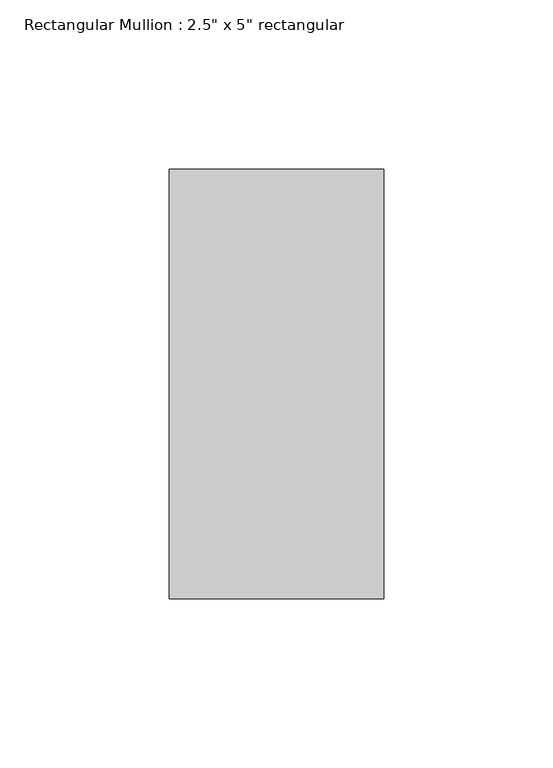
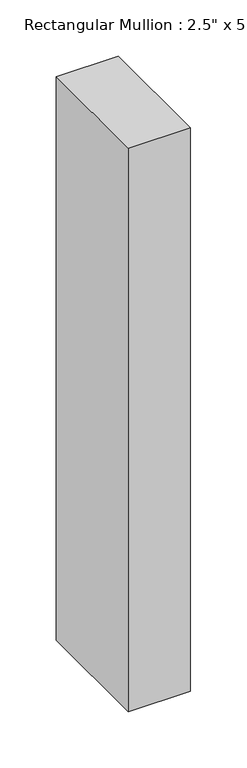
"""IFC4 building model written with IfcOpenShell, lengths in millimetres: member geometry."""

from ifc_helpers import new_model, si_unit, frame, origin, place, context, project, spatial, polyline, outline, extrude, source, transform, mapped, element, save


def member_6e77e263(model_context):
    return source(origin(), model_context, "Body", "SweptSolid", [
        extrude(outline(polyline([(31.75, 63.5), (31.75, -63.5), (-31.75, -63.5), (-31.75, 63.5), (31.75, 63.5)])), frame((0.0, 0.0, -609.6), z_axis=(0.0, 0.0, 1.0), x_axis=(1.0, 0.0, 0.0)), (0.0, 0.0, 1.0), 609.6),
    ])


if __name__ == "__main__":
    model = new_model("IFC4")
    model_context = context("Model", 3, world=origin())
    ifc_project = project(units=[si_unit("LENGTHUNIT", "METRE", prefix="MILLI")], contexts=[model_context])
    site = spatial("IfcSite", under=ifc_project)
    building = spatial("IfcBuilding", under=site)
    placement = place(None, origin())
    member_shape = member_6e77e263(model_context)
    element("IfcMember", 1, ObjectType="Rectangular Mullion : 2.5\" x 5\" rectangular", at=placement, inside=building, context=model_context, shape_type="MappedRepresentation", body=[
        mapped(member_shape, transform((0.0, 0.0, 0.0), x_axis=(1.0, 0.0, 0.0), y_axis=(0.0, 1.0, 0.0), z_axis=(0.0, 0.0, 1.0))),
    ])
    save(model, "model.ifc")

# Revit data of these elements
# Type "Rectangular Mullion : 2.5\" x 5\" rectangular"
#   built-in parameter 1007304 = 0.416667 (stored number, unit not read)
#   built-in parameter 1007301 = 0.104167 (stored number, unit not read)
#   built-in parameter 1007300 = 0.104167 (stored number, unit not read)
# Element 1 (IfcMember, "Rectangular Mullion : 2.5\" x 5\" rectangular")
#   Materials on its faces: "metal black"
# Materials
#   "metal black": class "Generic", colour RGB 120 120 120, transparency 0, Cost = 0
